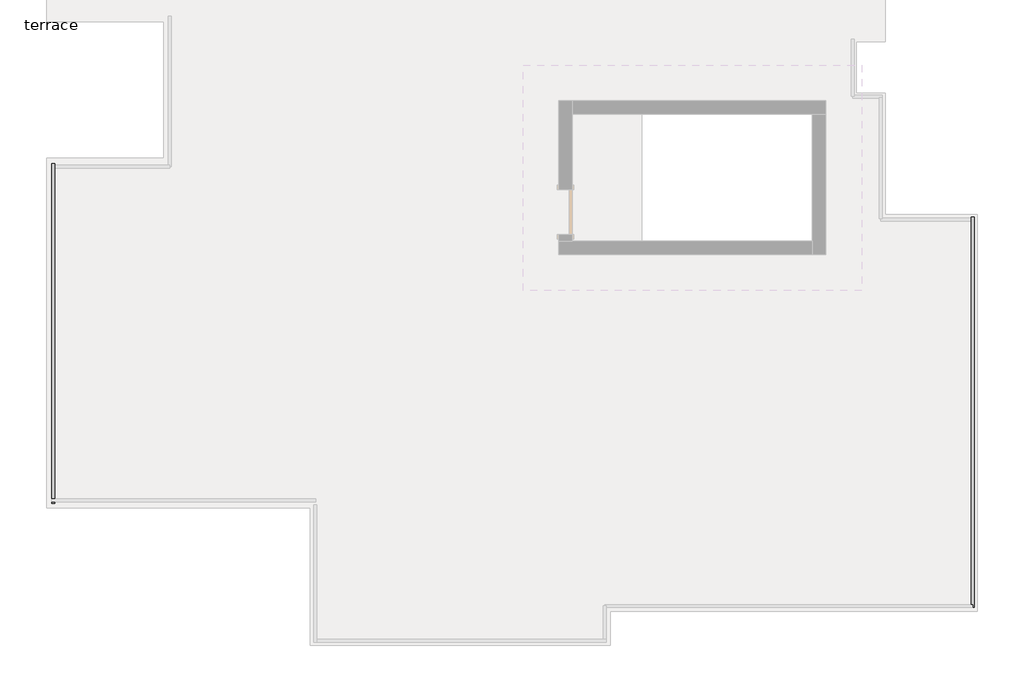
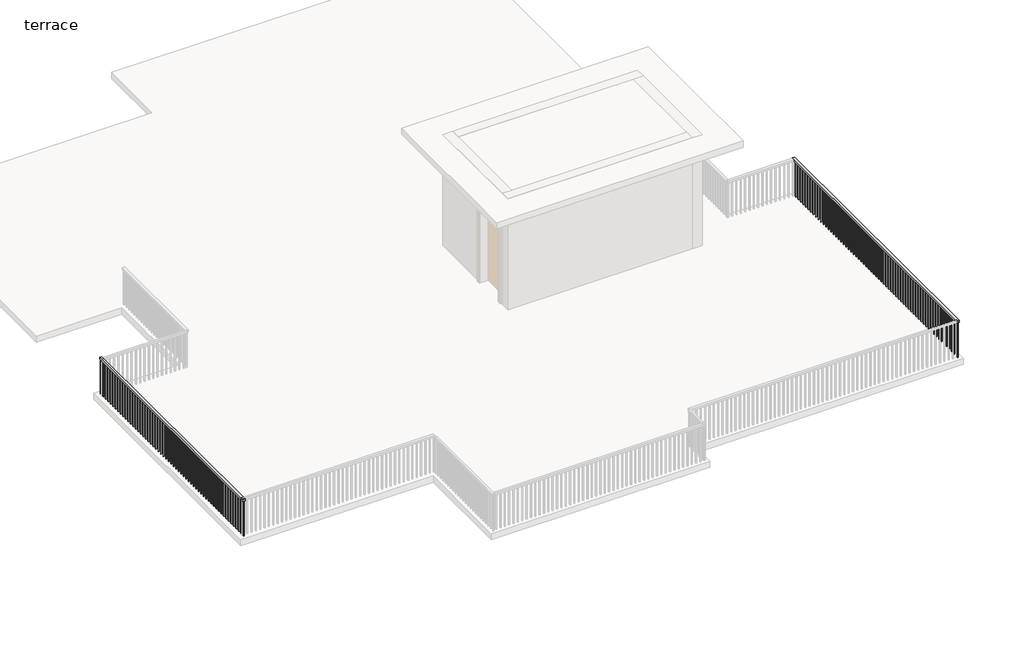
# One storey, part 3 of 7: 2 railings.
"""IFC4 building model written with IfcOpenShell, lengths in millimetres."""

from ifc_helpers import new_model, si_unit, frame, origin, place, context, project, spatial, polyline, outline, extrude, element, save

model = new_model("IFC4")

# Units and contexts
model_context = context("Model", 3, world=origin())
ifc_project = project(units=[si_unit("LENGTHUNIT", "METRE", prefix="MILLI")], contexts=[model_context])

# Site, building, storey
site = spatial("IfcSite", under=ifc_project)
building = spatial("IfcBuilding", under=site)
storey = spatial("IfcBuildingStorey", under=building, Name="terrace", Elevation=3810.0)

# Railings
placement = place(None, origin())
element("IfcRailing", 1, ObjectType="Handrail - Rectangular", at=placement, inside=storey, context=model_context, shape_type="SweptSolid", body=[
    extrude(outline(polyline([(1267.5109871, 2105.327622), (1318.3109871, 2105.327622), (1318.3109871, -4549.472378), (1267.5109871, -4549.472378), (1267.5109871, 2105.327622)])), frame((0.0, 0.0, 4673.6), z_axis=(0.0, 0.0, 1.0), x_axis=(1.0, 0.0, 0.0)), (0.0, 0.0, 1.0), 50.8),
    extrude(outline(polyline([(1283.3859871, -4489.147378), (1302.4359871, -4489.147378), (1302.4359871, -4508.197378), (1283.3859871, -4508.197378), (1283.3859871, -4489.147378)])), frame((0.0, 0.0, 3810.0), z_axis=(0.0, 0.0, 1.0), x_axis=(1.0, 0.0, 0.0)), (0.0, 0.0, 1.0), 863.6),
    extrude(outline(polyline([(1283.3859871, -4387.547378), (1302.4359871, -4387.547378), (1302.4359871, -4406.597378), (1283.3859871, -4406.597378), (1283.3859871, -4387.547378)])), frame((0.0, 0.0, 3810.0), z_axis=(0.0, 0.0, 1.0), x_axis=(1.0, 0.0, 0.0)), (0.0, 0.0, 1.0), 863.6),
    extrude(outline(polyline([(1283.3859871, -4285.947378), (1302.4359871, -4285.947378), (1302.4359871, -4304.997378), (1283.3859871, -4304.997378), (1283.3859871, -4285.947378)])), frame((0.0, 0.0, 3810.0), z_axis=(0.0, 0.0, 1.0), x_axis=(1.0, 0.0, 0.0)), (0.0, 0.0, 1.0), 863.6),
    extrude(outline(polyline([(1283.3859871, -4184.347378), (1302.4359871, -4184.347378), (1302.4359871, -4203.397378), (1283.3859871, -4203.397378), (1283.3859871, -4184.347378)])), frame((0.0, 0.0, 3810.0), z_axis=(0.0, 0.0, 1.0), x_axis=(1.0, 0.0, 0.0)), (0.0, 0.0, 1.0), 863.6),
    extrude(outline(polyline([(1283.3859871, -4082.747378), (1302.4359871, -4082.747378), (1302.4359871, -4101.797378), (1283.3859871, -4101.797378), (1283.3859871, -4082.747378)])), frame((0.0, 0.0, 3810.0), z_axis=(0.0, 0.0, 1.0), x_axis=(1.0, 0.0, 0.0)), (0.0, 0.0, 1.0), 863.6),
    extrude(outline(polyline([(1283.3859871, -3981.147378), (1302.4359871, -3981.147378), (1302.4359871, -4000.197378), (1283.3859871, -4000.197378), (1283.3859871, -3981.147378)])), frame((0.0, 0.0, 3810.0), z_axis=(0.0, 0.0, 1.0), x_axis=(1.0, 0.0, 0.0)), (0.0, 0.0, 1.0), 863.6),
    extrude(outline(polyline([(1283.3859871, -3879.547378), (1302.4359871, -3879.547378), (1302.4359871, -3898.597378), (1283.3859871, -3898.597378), (1283.3859871, -3879.547378)])), frame((0.0, 0.0, 3810.0), z_axis=(0.0, 0.0, 1.0), x_axis=(1.0, 0.0, 0.0)), (0.0, 0.0, 1.0), 863.6),
    extrude(outline(polyline([(1283.3859871, -3777.947378), (1302.4359871, -3777.947378), (1302.4359871, -3796.997378), (1283.3859871, -3796.997378), (1283.3859871, -3777.947378)])), frame((0.0, 0.0, 3810.0), z_axis=(0.0, 0.0, 1.0), x_axis=(1.0, 0.0, 0.0)), (0.0, 0.0, 1.0), 863.6),
    extrude(outline(polyline([(1283.3859871, -3676.347378), (1302.4359871, -3676.347378), (1302.4359871, -3695.397378), (1283.3859871, -3695.397378), (1283.3859871, -3676.347378)])), frame((0.0, 0.0, 3810.0), z_axis=(0.0, 0.0, 1.0), x_axis=(1.0, 0.0, 0.0)), (0.0, 0.0, 1.0), 863.6),
    extrude(outline(polyline([(1283.3859871, -3574.747378), (1302.4359871, -3574.747378), (1302.4359871, -3593.797378), (1283.3859871, -3593.797378), (1283.3859871, -3574.747378)])), frame((0.0, 0.0, 3810.0), z_axis=(0.0, 0.0, 1.0), x_axis=(1.0, 0.0, 0.0)), (0.0, 0.0, 1.0), 863.6),
    extrude(outline(polyline([(1283.3859871, -3473.147378), (1302.4359871, -3473.147378), (1302.4359871, -3492.197378), (1283.3859871, -3492.197378), (1283.3859871, -3473.147378)])), frame((0.0, 0.0, 3810.0), z_axis=(0.0, 0.0, 1.0), x_axis=(1.0, 0.0, 0.0)), (0.0, 0.0, 1.0), 863.6),
    extrude(outline(polyline([(1283.3859871, -3371.547378), (1302.4359871, -3371.547378), (1302.4359871, -3390.597378), (1283.3859871, -3390.597378), (1283.3859871, -3371.547378)])), frame((0.0, 0.0, 3810.0), z_axis=(0.0, 0.0, 1.0), x_axis=(1.0, 0.0, 0.0)), (0.0, 0.0, 1.0), 863.6),
    extrude(outline(polyline([(1283.3859871, -3269.947378), (1302.4359871, -3269.947378), (1302.4359871, -3288.997378), (1283.3859871, -3288.997378), (1283.3859871, -3269.947378)])), frame((0.0, 0.0, 3810.0), z_axis=(0.0, 0.0, 1.0), x_axis=(1.0, 0.0, 0.0)), (0.0, 0.0, 1.0), 863.6),
    extrude(outline(polyline([(1283.3859871, -3168.347378), (1302.4359871, -3168.347378), (1302.4359871, -3187.397378), (1283.3859871, -3187.397378), (1283.3859871, -3168.347378)])), frame((0.0, 0.0, 3810.0), z_axis=(0.0, 0.0, 1.0), x_axis=(1.0, 0.0, 0.0)), (0.0, 0.0, 1.0), 863.6),
    extrude(outline(polyline([(1283.3859871, -3066.747378), (1302.4359871, -3066.747378), (1302.4359871, -3085.797378), (1283.3859871, -3085.797378), (1283.3859871, -3066.747378)])), frame((0.0, 0.0, 3810.0), z_axis=(0.0, 0.0, 1.0), x_axis=(1.0, 0.0, 0.0)), (0.0, 0.0, 1.0), 863.6),
    extrude(outline(polyline([(1283.3859871, -2965.147378), (1302.4359871, -2965.147378), (1302.4359871, -2984.197378), (1283.3859871, -2984.197378), (1283.3859871, -2965.147378)])), frame((0.0, 0.0, 3810.0), z_axis=(0.0, 0.0, 1.0), x_axis=(1.0, 0.0, 0.0)), (0.0, 0.0, 1.0), 863.6),
    extrude(outline(polyline([(1283.3859871, -2863.547378), (1302.4359871, -2863.547378), (1302.4359871, -2882.597378), (1283.3859871, -2882.597378), (1283.3859871, -2863.547378)])), frame((0.0, 0.0, 3810.0), z_axis=(0.0, 0.0, 1.0), x_axis=(1.0, 0.0, 0.0)), (0.0, 0.0, 1.0), 863.6),
    extrude(outline(polyline([(1283.3859871, -2761.947378), (1302.4359871, -2761.947378), (1302.4359871, -2780.997378), (1283.3859871, -2780.997378), (1283.3859871, -2761.947378)])), frame((0.0, 0.0, 3810.0), z_axis=(0.0, 0.0, 1.0), x_axis=(1.0, 0.0, 0.0)), (0.0, 0.0, 1.0), 863.6),
    extrude(outline(polyline([(1283.3859871, -2660.347378), (1302.4359871, -2660.347378), (1302.4359871, -2679.397378), (1283.3859871, -2679.397378), (1283.3859871, -2660.347378)])), frame((0.0, 0.0, 3810.0), z_axis=(0.0, 0.0, 1.0), x_axis=(1.0, 0.0, 0.0)), (0.0, 0.0, 1.0), 863.6),
    extrude(outline(polyline([(1283.3859871, -2558.747378), (1302.4359871, -2558.747378), (1302.4359871, -2577.797378), (1283.3859871, -2577.797378), (1283.3859871, -2558.747378)])), frame((0.0, 0.0, 3810.0), z_axis=(0.0, 0.0, 1.0), x_axis=(1.0, 0.0, 0.0)), (0.0, 0.0, 1.0), 863.6),
    extrude(outline(polyline([(1283.3859871, -2457.147378), (1302.4359871, -2457.147378), (1302.4359871, -2476.197378), (1283.3859871, -2476.197378), (1283.3859871, -2457.147378)])), frame((0.0, 0.0, 3810.0), z_axis=(0.0, 0.0, 1.0), x_axis=(1.0, 0.0, 0.0)), (0.0, 0.0, 1.0), 863.6),
    extrude(outline(polyline([(1283.3859871, -2355.547378), (1302.4359871, -2355.547378), (1302.4359871, -2374.597378), (1283.3859871, -2374.597378), (1283.3859871, -2355.547378)])), frame((0.0, 0.0, 3810.0), z_axis=(0.0, 0.0, 1.0), x_axis=(1.0, 0.0, 0.0)), (0.0, 0.0, 1.0), 863.6),
    extrude(outline(polyline([(1283.3859871, -2253.947378), (1302.4359871, -2253.947378), (1302.4359871, -2272.997378), (1283.3859871, -2272.997378), (1283.3859871, -2253.947378)])), frame((0.0, 0.0, 3810.0), z_axis=(0.0, 0.0, 1.0), x_axis=(1.0, 0.0, 0.0)), (0.0, 0.0, 1.0), 863.6),
    extrude(outline(polyline([(1283.3859871, -2152.347378), (1302.4359871, -2152.347378), (1302.4359871, -2171.397378), (1283.3859871, -2171.397378), (1283.3859871, -2152.347378)])), frame((0.0, 0.0, 3810.0), z_axis=(0.0, 0.0, 1.0), x_axis=(1.0, 0.0, 0.0)), (0.0, 0.0, 1.0), 863.6),
    extrude(outline(polyline([(1283.3859871, -2050.747378), (1302.4359871, -2050.747378), (1302.4359871, -2069.797378), (1283.3859871, -2069.797378), (1283.3859871, -2050.747378)])), frame((0.0, 0.0, 3810.0), z_axis=(0.0, 0.0, 1.0), x_axis=(1.0, 0.0, 0.0)), (0.0, 0.0, 1.0), 863.6),
    extrude(outline(polyline([(1283.3859871, -1949.147378), (1302.4359871, -1949.147378), (1302.4359871, -1968.197378), (1283.3859871, -1968.197378), (1283.3859871, -1949.147378)])), frame((0.0, 0.0, 3810.0), z_axis=(0.0, 0.0, 1.0), x_axis=(1.0, 0.0, 0.0)), (0.0, 0.0, 1.0), 863.6),
    extrude(outline(polyline([(1283.3859871, -1847.547378), (1302.4359871, -1847.547378), (1302.4359871, -1866.597378), (1283.3859871, -1866.597378), (1283.3859871, -1847.547378)])), frame((0.0, 0.0, 3810.0), z_axis=(0.0, 0.0, 1.0), x_axis=(1.0, 0.0, 0.0)), (0.0, 0.0, 1.0), 863.6),
    extrude(outline(polyline([(1283.3859871, -1745.947378), (1302.4359871, -1745.947378), (1302.4359871, -1764.997378), (1283.3859871, -1764.997378), (1283.3859871, -1745.947378)])), frame((0.0, 0.0, 3810.0), z_axis=(0.0, 0.0, 1.0), x_axis=(1.0, 0.0, 0.0)), (0.0, 0.0, 1.0), 863.6),
    extrude(outline(polyline([(1283.3859871, -1644.347378), (1302.4359871, -1644.347378), (1302.4359871, -1663.397378), (1283.3859871, -1663.397378), (1283.3859871, -1644.347378)])), frame((0.0, 0.0, 3810.0), z_axis=(0.0, 0.0, 1.0), x_axis=(1.0, 0.0, 0.0)), (0.0, 0.0, 1.0), 863.6),
    extrude(outline(polyline([(1283.3859871, -1542.747378), (1302.4359871, -1542.747378), (1302.4359871, -1561.797378), (1283.3859871, -1561.797378), (1283.3859871, -1542.747378)])), frame((0.0, 0.0, 3810.0), z_axis=(0.0, 0.0, 1.0), x_axis=(1.0, 0.0, 0.0)), (0.0, 0.0, 1.0), 863.6),
    extrude(outline(polyline([(1283.3859871, -1441.147378), (1302.4359871, -1441.147378), (1302.4359871, -1460.197378), (1283.3859871, -1460.197378), (1283.3859871, -1441.147378)])), frame((0.0, 0.0, 3810.0), z_axis=(0.0, 0.0, 1.0), x_axis=(1.0, 0.0, 0.0)), (0.0, 0.0, 1.0), 863.6),
    extrude(outline(polyline([(1283.3859871, -1339.547378), (1302.4359871, -1339.547378), (1302.4359871, -1358.597378), (1283.3859871, -1358.597378), (1283.3859871, -1339.547378)])), frame((0.0, 0.0, 3810.0), z_axis=(0.0, 0.0, 1.0), x_axis=(1.0, 0.0, 0.0)), (0.0, 0.0, 1.0), 863.6),
    extrude(outline(polyline([(1283.3859871, -1237.947378), (1302.4359871, -1237.947378), (1302.4359871, -1256.997378), (1283.3859871, -1256.997378), (1283.3859871, -1237.947378)])), frame((0.0, 0.0, 3810.0), z_axis=(0.0, 0.0, 1.0), x_axis=(1.0, 0.0, 0.0)), (0.0, 0.0, 1.0), 863.6),
    extrude(outline(polyline([(1283.3859871, -1136.347378), (1302.4359871, -1136.347378), (1302.4359871, -1155.397378), (1283.3859871, -1155.397378), (1283.3859871, -1136.347378)])), frame((0.0, 0.0, 3810.0), z_axis=(0.0, 0.0, 1.0), x_axis=(1.0, 0.0, 0.0)), (0.0, 0.0, 1.0), 863.6),
    extrude(outline(polyline([(1283.3859871, -1034.747378), (1302.4359871, -1034.747378), (1302.4359871, -1053.797378), (1283.3859871, -1053.797378), (1283.3859871, -1034.747378)])), frame((0.0, 0.0, 3810.0), z_axis=(0.0, 0.0, 1.0), x_axis=(1.0, 0.0, 0.0)), (0.0, 0.0, 1.0), 863.6),
    extrude(outline(polyline([(1283.3859871, -933.147378), (1302.4359871, -933.147378), (1302.4359871, -952.197378), (1283.3859871, -952.197378), (1283.3859871, -933.147378)])), frame((0.0, 0.0, 3810.0), z_axis=(0.0, 0.0, 1.0), x_axis=(1.0, 0.0, 0.0)), (0.0, 0.0, 1.0), 863.6),
    extrude(outline(polyline([(1283.3859871, -831.547378), (1302.4359871, -831.547378), (1302.4359871, -850.597378), (1283.3859871, -850.597378), (1283.3859871, -831.547378)])), frame((0.0, 0.0, 3810.0), z_axis=(0.0, 0.0, 1.0), x_axis=(1.0, 0.0, 0.0)), (0.0, 0.0, 1.0), 863.6),
    extrude(outline(polyline([(1283.3859871, -729.947378), (1302.4359871, -729.947378), (1302.4359871, -748.997378), (1283.3859871, -748.997378), (1283.3859871, -729.947378)])), frame((0.0, 0.0, 3810.0), z_axis=(0.0, 0.0, 1.0), x_axis=(1.0, 0.0, 0.0)), (0.0, 0.0, 1.0), 863.6),
    extrude(outline(polyline([(1283.3859871, -628.347378), (1302.4359871, -628.347378), (1302.4359871, -647.397378), (1283.3859871, -647.397378), (1283.3859871, -628.347378)])), frame((0.0, 0.0, 3810.0), z_axis=(0.0, 0.0, 1.0), x_axis=(1.0, 0.0, 0.0)), (0.0, 0.0, 1.0), 863.6),
    extrude(outline(polyline([(1283.3859871, -526.747378), (1302.4359871, -526.747378), (1302.4359871, -545.797378), (1283.3859871, -545.797378), (1283.3859871, -526.747378)])), frame((0.0, 0.0, 3810.0), z_axis=(0.0, 0.0, 1.0), x_axis=(1.0, 0.0, 0.0)), (0.0, 0.0, 1.0), 863.6),
    extrude(outline(polyline([(1283.3859871, -425.147378), (1302.4359871, -425.147378), (1302.4359871, -444.197378), (1283.3859871, -444.197378), (1283.3859871, -425.147378)])), frame((0.0, 0.0, 3810.0), z_axis=(0.0, 0.0, 1.0), x_axis=(1.0, 0.0, 0.0)), (0.0, 0.0, 1.0), 863.6),
    extrude(outline(polyline([(1283.3859871, -323.547378), (1302.4359871, -323.547378), (1302.4359871, -342.597378), (1283.3859871, -342.597378), (1283.3859871, -323.547378)])), frame((0.0, 0.0, 3810.0), z_axis=(0.0, 0.0, 1.0), x_axis=(1.0, 0.0, 0.0)), (0.0, 0.0, 1.0), 863.6),
    extrude(outline(polyline([(1283.3859871, -221.947378), (1302.4359871, -221.947378), (1302.4359871, -240.997378), (1283.3859871, -240.997378), (1283.3859871, -221.947378)])), frame((0.0, 0.0, 3810.0), z_axis=(0.0, 0.0, 1.0), x_axis=(1.0, 0.0, 0.0)), (0.0, 0.0, 1.0), 863.6),
    extrude(outline(polyline([(1283.3859871, -120.347378), (1302.4359871, -120.347378), (1302.4359871, -139.397378), (1283.3859871, -139.397378), (1283.3859871, -120.347378)])), frame((0.0, 0.0, 3810.0), z_axis=(0.0, 0.0, 1.0), x_axis=(1.0, 0.0, 0.0)), (0.0, 0.0, 1.0), 863.6),
    extrude(outline(polyline([(1283.3859871, -18.747378), (1302.4359871, -18.747378), (1302.4359871, -37.797378), (1283.3859871, -37.797378), (1283.3859871, -18.747378)])), frame((0.0, 0.0, 3810.0), z_axis=(0.0, 0.0, 1.0), x_axis=(1.0, 0.0, 0.0)), (0.0, 0.0, 1.0), 863.6),
    extrude(outline(polyline([(1283.3859871, 82.852622), (1302.4359871, 82.852622), (1302.4359871, 63.802622), (1283.3859871, 63.802622), (1283.3859871, 82.852622)])), frame((0.0, 0.0, 3810.0), z_axis=(0.0, 0.0, 1.0), x_axis=(1.0, 0.0, 0.0)), (0.0, 0.0, 1.0), 863.6),
    extrude(outline(polyline([(1283.3859871, 184.452622), (1302.4359871, 184.452622), (1302.4359871, 165.402622), (1283.3859871, 165.402622), (1283.3859871, 184.452622)])), frame((0.0, 0.0, 3810.0), z_axis=(0.0, 0.0, 1.0), x_axis=(1.0, 0.0, 0.0)), (0.0, 0.0, 1.0), 863.6),
    extrude(outline(polyline([(1283.3859871, 286.052622), (1302.4359871, 286.052622), (1302.4359871, 267.002622), (1283.3859871, 267.002622), (1283.3859871, 286.052622)])), frame((0.0, 0.0, 3810.0), z_axis=(0.0, 0.0, 1.0), x_axis=(1.0, 0.0, 0.0)), (0.0, 0.0, 1.0), 863.6),
    extrude(outline(polyline([(1283.3859871, 387.652622), (1302.4359871, 387.652622), (1302.4359871, 368.602622), (1283.3859871, 368.602622), (1283.3859871, 387.652622)])), frame((0.0, 0.0, 3810.0), z_axis=(0.0, 0.0, 1.0), x_axis=(1.0, 0.0, 0.0)), (0.0, 0.0, 1.0), 863.6),
    extrude(outline(polyline([(1283.3859871, 489.252622), (1302.4359871, 489.252622), (1302.4359871, 470.202622), (1283.3859871, 470.202622), (1283.3859871, 489.252622)])), frame((0.0, 0.0, 3810.0), z_axis=(0.0, 0.0, 1.0), x_axis=(1.0, 0.0, 0.0)), (0.0, 0.0, 1.0), 863.6),
    extrude(outline(polyline([(1283.3859871, 590.852622), (1302.4359871, 590.852622), (1302.4359871, 571.802622), (1283.3859871, 571.802622), (1283.3859871, 590.852622)])), frame((0.0, 0.0, 3810.0), z_axis=(0.0, 0.0, 1.0), x_axis=(1.0, 0.0, 0.0)), (0.0, 0.0, 1.0), 863.6),
    extrude(outline(polyline([(1283.3859871, 692.452622), (1302.4359871, 692.452622), (1302.4359871, 673.402622), (1283.3859871, 673.402622), (1283.3859871, 692.452622)])), frame((0.0, 0.0, 3810.0), z_axis=(0.0, 0.0, 1.0), x_axis=(1.0, 0.0, 0.0)), (0.0, 0.0, 1.0), 863.6),
    extrude(outline(polyline([(1283.3859871, 794.052622), (1302.4359871, 794.052622), (1302.4359871, 775.002622), (1283.3859871, 775.002622), (1283.3859871, 794.052622)])), frame((0.0, 0.0, 3810.0), z_axis=(0.0, 0.0, 1.0), x_axis=(1.0, 0.0, 0.0)), (0.0, 0.0, 1.0), 863.6),
    extrude(outline(polyline([(1283.3859871, 895.652622), (1302.4359871, 895.652622), (1302.4359871, 876.602622), (1283.3859871, 876.602622), (1283.3859871, 895.652622)])), frame((0.0, 0.0, 3810.0), z_axis=(0.0, 0.0, 1.0), x_axis=(1.0, 0.0, 0.0)), (0.0, 0.0, 1.0), 863.6),
    extrude(outline(polyline([(1283.3859871, 997.252622), (1302.4359871, 997.252622), (1302.4359871, 978.202622), (1283.3859871, 978.202622), (1283.3859871, 997.252622)])), frame((0.0, 0.0, 3810.0), z_axis=(0.0, 0.0, 1.0), x_axis=(1.0, 0.0, 0.0)), (0.0, 0.0, 1.0), 863.6),
    extrude(outline(polyline([(1283.3859871, 1098.852622), (1302.4359871, 1098.852622), (1302.4359871, 1079.802622), (1283.3859871, 1079.802622), (1283.3859871, 1098.852622)])), frame((0.0, 0.0, 3810.0), z_axis=(0.0, 0.0, 1.0), x_axis=(1.0, 0.0, 0.0)), (0.0, 0.0, 1.0), 863.6),
    extrude(outline(polyline([(1283.3859871, 1200.452622), (1302.4359871, 1200.452622), (1302.4359871, 1181.402622), (1283.3859871, 1181.402622), (1283.3859871, 1200.452622)])), frame((0.0, 0.0, 3810.0), z_axis=(0.0, 0.0, 1.0), x_axis=(1.0, 0.0, 0.0)), (0.0, 0.0, 1.0), 863.6),
    extrude(outline(polyline([(1283.3859871, 1302.052622), (1302.4359871, 1302.052622), (1302.4359871, 1283.002622), (1283.3859871, 1283.002622), (1283.3859871, 1302.052622)])), frame((0.0, 0.0, 3810.0), z_axis=(0.0, 0.0, 1.0), x_axis=(1.0, 0.0, 0.0)), (0.0, 0.0, 1.0), 863.6),
    extrude(outline(polyline([(1283.3859871, 1403.652622), (1302.4359871, 1403.652622), (1302.4359871, 1384.602622), (1283.3859871, 1384.602622), (1283.3859871, 1403.652622)])), frame((0.0, 0.0, 3810.0), z_axis=(0.0, 0.0, 1.0), x_axis=(1.0, 0.0, 0.0)), (0.0, 0.0, 1.0), 863.6),
    extrude(outline(polyline([(1283.3859871, 1505.252622), (1302.4359871, 1505.252622), (1302.4359871, 1486.202622), (1283.3859871, 1486.202622), (1283.3859871, 1505.252622)])), frame((0.0, 0.0, 3810.0), z_axis=(0.0, 0.0, 1.0), x_axis=(1.0, 0.0, 0.0)), (0.0, 0.0, 1.0), 863.6),
    extrude(outline(polyline([(1283.3859871, 1606.852622), (1302.4359871, 1606.852622), (1302.4359871, 1587.802622), (1283.3859871, 1587.802622), (1283.3859871, 1606.852622)])), frame((0.0, 0.0, 3810.0), z_axis=(0.0, 0.0, 1.0), x_axis=(1.0, 0.0, 0.0)), (0.0, 0.0, 1.0), 863.6),
    extrude(outline(polyline([(1283.3859871, 1708.452622), (1302.4359871, 1708.452622), (1302.4359871, 1689.402622), (1283.3859871, 1689.402622), (1283.3859871, 1708.452622)])), frame((0.0, 0.0, 3810.0), z_axis=(0.0, 0.0, 1.0), x_axis=(1.0, 0.0, 0.0)), (0.0, 0.0, 1.0), 863.6),
    extrude(outline(polyline([(1283.3859871, 1810.052622), (1302.4359871, 1810.052622), (1302.4359871, 1791.002622), (1283.3859871, 1791.002622), (1283.3859871, 1810.052622)])), frame((0.0, 0.0, 3810.0), z_axis=(0.0, 0.0, 1.0), x_axis=(1.0, 0.0, 0.0)), (0.0, 0.0, 1.0), 863.6),
    extrude(outline(polyline([(1283.3859871, 1911.652622), (1302.4359871, 1911.652622), (1302.4359871, 1892.602622), (1283.3859871, 1892.602622), (1283.3859871, 1911.652622)])), frame((0.0, 0.0, 3810.0), z_axis=(0.0, 0.0, 1.0), x_axis=(1.0, 0.0, 0.0)), (0.0, 0.0, 1.0), 863.6),
    extrude(outline(polyline([(1283.3859871, 2013.252622), (1302.4359871, 2013.252622), (1302.4359871, 1994.202622), (1283.3859871, 1994.202622), (1283.3859871, 2013.252622)])), frame((0.0, 0.0, 3810.0), z_axis=(0.0, 0.0, 1.0), x_axis=(1.0, 0.0, 0.0)), (0.0, 0.0, 1.0), 863.6),
    extrude(outline(polyline([(1283.3859871, -4530.422378), (1302.4359871, -4530.422378), (1302.4359871, -4549.472378), (1283.3859871, -4549.472378), (1283.3859871, -4530.422378)])), frame((0.0, 0.0, 3810.0), z_axis=(0.0, 0.0, 1.0), x_axis=(1.0, 0.0, 0.0)), (0.0, 0.0, 1.0), 863.6),
    extrude(outline(polyline([(1283.3859871, 2105.327622), (1302.4359871, 2105.327622), (1302.4359871, 2086.277622), (1283.3859871, 2086.277622), (1283.3859871, 2105.327622)])), frame((0.0, 0.0, 3810.0), z_axis=(0.0, 0.0, 1.0), x_axis=(1.0, 0.0, 0.0)), (0.0, 0.0, 1.0), 863.6),
])
element("IfcRailing", 2, ObjectType="Handrail - Rectangular", at=placement, inside=storey, context=model_context, shape_type="SweptSolid", body=[
    extrude(outline(polyline([(-14340.7890129, -2777.822378), (-14391.5890129, -2777.822378), (-14391.5890129, 3013.377622), (-14340.7890129, 3013.377622), (-14340.7890129, -2777.822378)])), frame((0.0, 0.0, 4673.6), z_axis=(0.0, 0.0, 1.0), x_axis=(1.0, 0.0, 0.0)), (0.0, 0.0, 1.0), 50.8),
    extrude(outline(polyline([(-14356.6640129, 2902.252622), (-14375.7140129, 2902.252622), (-14375.7140129, 2921.302622), (-14356.6640129, 2921.302622), (-14356.6640129, 2902.252622)])), frame((0.0, 0.0, 3810.0), z_axis=(0.0, 0.0, 1.0), x_axis=(1.0, 0.0, 0.0)), (0.0, 0.0, 1.0), 863.6),
    extrude(outline(polyline([(-14356.6640129, 2800.652622), (-14375.7140129, 2800.652622), (-14375.7140129, 2819.702622), (-14356.6640129, 2819.702622), (-14356.6640129, 2800.652622)])), frame((0.0, 0.0, 3810.0), z_axis=(0.0, 0.0, 1.0), x_axis=(1.0, 0.0, 0.0)), (0.0, 0.0, 1.0), 863.6),
    extrude(outline(polyline([(-14356.6640129, 2699.052622), (-14375.7140129, 2699.052622), (-14375.7140129, 2718.102622), (-14356.6640129, 2718.102622), (-14356.6640129, 2699.052622)])), frame((0.0, 0.0, 3810.0), z_axis=(0.0, 0.0, 1.0), x_axis=(1.0, 0.0, 0.0)), (0.0, 0.0, 1.0), 863.6),
    extrude(outline(polyline([(-14356.6640129, 2597.452622), (-14375.7140129, 2597.452622), (-14375.7140129, 2616.502622), (-14356.6640129, 2616.502622), (-14356.6640129, 2597.452622)])), frame((0.0, 0.0, 3810.0), z_axis=(0.0, 0.0, 1.0), x_axis=(1.0, 0.0, 0.0)), (0.0, 0.0, 1.0), 863.6),
    extrude(outline(polyline([(-14356.6640129, 2495.852622), (-14375.7140129, 2495.852622), (-14375.7140129, 2514.902622), (-14356.6640129, 2514.902622), (-14356.6640129, 2495.852622)])), frame((0.0, 0.0, 3810.0), z_axis=(0.0, 0.0, 1.0), x_axis=(1.0, 0.0, 0.0)), (0.0, 0.0, 1.0), 863.6),
    extrude(outline(polyline([(-14356.6640129, 2394.252622), (-14375.7140129, 2394.252622), (-14375.7140129, 2413.302622), (-14356.6640129, 2413.302622), (-14356.6640129, 2394.252622)])), frame((0.0, 0.0, 3810.0), z_axis=(0.0, 0.0, 1.0), x_axis=(1.0, 0.0, 0.0)), (0.0, 0.0, 1.0), 863.6),
    extrude(outline(polyline([(-14356.6640129, 2292.652622), (-14375.7140129, 2292.652622), (-14375.7140129, 2311.702622), (-14356.6640129, 2311.702622), (-14356.6640129, 2292.652622)])), frame((0.0, 0.0, 3810.0), z_axis=(0.0, 0.0, 1.0), x_axis=(1.0, 0.0, 0.0)), (0.0, 0.0, 1.0), 863.6),
    extrude(outline(polyline([(-14356.6640129, 2191.052622), (-14375.7140129, 2191.052622), (-14375.7140129, 2210.102622), (-14356.6640129, 2210.102622), (-14356.6640129, 2191.052622)])), frame((0.0, 0.0, 3810.0), z_axis=(0.0, 0.0, 1.0), x_axis=(1.0, 0.0, 0.0)), (0.0, 0.0, 1.0), 863.6),
    extrude(outline(polyline([(-14356.6640129, 2089.452622), (-14375.7140129, 2089.452622), (-14375.7140129, 2108.502622), (-14356.6640129, 2108.502622), (-14356.6640129, 2089.452622)])), frame((0.0, 0.0, 3810.0), z_axis=(0.0, 0.0, 1.0), x_axis=(1.0, 0.0, 0.0)), (0.0, 0.0, 1.0), 863.6),
    extrude(outline(polyline([(-14356.6640129, 1987.852622), (-14375.7140129, 1987.852622), (-14375.7140129, 2006.902622), (-14356.6640129, 2006.902622), (-14356.6640129, 1987.852622)])), frame((0.0, 0.0, 3810.0), z_axis=(0.0, 0.0, 1.0), x_axis=(1.0, 0.0, 0.0)), (0.0, 0.0, 1.0), 863.6),
    extrude(outline(polyline([(-14356.6640129, 1886.252622), (-14375.7140129, 1886.252622), (-14375.7140129, 1905.302622), (-14356.6640129, 1905.302622), (-14356.6640129, 1886.252622)])), frame((0.0, 0.0, 3810.0), z_axis=(0.0, 0.0, 1.0), x_axis=(1.0, 0.0, 0.0)), (0.0, 0.0, 1.0), 863.6),
    extrude(outline(polyline([(-14356.6640129, 1784.652622), (-14375.7140129, 1784.652622), (-14375.7140129, 1803.702622), (-14356.6640129, 1803.702622), (-14356.6640129, 1784.652622)])), frame((0.0, 0.0, 3810.0), z_axis=(0.0, 0.0, 1.0), x_axis=(1.0, 0.0, 0.0)), (0.0, 0.0, 1.0), 863.6),
    extrude(outline(polyline([(-14356.6640129, 1683.052622), (-14375.7140129, 1683.052622), (-14375.7140129, 1702.102622), (-14356.6640129, 1702.102622), (-14356.6640129, 1683.052622)])), frame((0.0, 0.0, 3810.0), z_axis=(0.0, 0.0, 1.0), x_axis=(1.0, 0.0, 0.0)), (0.0, 0.0, 1.0), 863.6),
    extrude(outline(polyline([(-14356.6640129, 1581.452622), (-14375.7140129, 1581.452622), (-14375.7140129, 1600.502622), (-14356.6640129, 1600.502622), (-14356.6640129, 1581.452622)])), frame((0.0, 0.0, 3810.0), z_axis=(0.0, 0.0, 1.0), x_axis=(1.0, 0.0, 0.0)), (0.0, 0.0, 1.0), 863.6),
    extrude(outline(polyline([(-14356.6640129, 1479.852622), (-14375.7140129, 1479.852622), (-14375.7140129, 1498.902622), (-14356.6640129, 1498.902622), (-14356.6640129, 1479.852622)])), frame((0.0, 0.0, 3810.0), z_axis=(0.0, 0.0, 1.0), x_axis=(1.0, 0.0, 0.0)), (0.0, 0.0, 1.0), 863.6),
    extrude(outline(polyline([(-14356.6640129, 1378.252622), (-14375.7140129, 1378.252622), (-14375.7140129, 1397.302622), (-14356.6640129, 1397.302622), (-14356.6640129, 1378.252622)])), frame((0.0, 0.0, 3810.0), z_axis=(0.0, 0.0, 1.0), x_axis=(1.0, 0.0, 0.0)), (0.0, 0.0, 1.0), 863.6),
    extrude(outline(polyline([(-14356.6640129, 1276.652622), (-14375.7140129, 1276.652622), (-14375.7140129, 1295.702622), (-14356.6640129, 1295.702622), (-14356.6640129, 1276.652622)])), frame((0.0, 0.0, 3810.0), z_axis=(0.0, 0.0, 1.0), x_axis=(1.0, 0.0, 0.0)), (0.0, 0.0, 1.0), 863.6),
    extrude(outline(polyline([(-14356.6640129, 1175.052622), (-14375.7140129, 1175.052622), (-14375.7140129, 1194.102622), (-14356.6640129, 1194.102622), (-14356.6640129, 1175.052622)])), frame((0.0, 0.0, 3810.0), z_axis=(0.0, 0.0, 1.0), x_axis=(1.0, 0.0, 0.0)), (0.0, 0.0, 1.0), 863.6),
    extrude(outline(polyline([(-14356.6640129, 1073.452622), (-14375.7140129, 1073.452622), (-14375.7140129, 1092.502622), (-14356.6640129, 1092.502622), (-14356.6640129, 1073.452622)])), frame((0.0, 0.0, 3810.0), z_axis=(0.0, 0.0, 1.0), x_axis=(1.0, 0.0, 0.0)), (0.0, 0.0, 1.0), 863.6),
    extrude(outline(polyline([(-14356.6640129, 971.852622), (-14375.7140129, 971.852622), (-14375.7140129, 990.902622), (-14356.6640129, 990.902622), (-14356.6640129, 971.852622)])), frame((0.0, 0.0, 3810.0), z_axis=(0.0, 0.0, 1.0), x_axis=(1.0, 0.0, 0.0)), (0.0, 0.0, 1.0), 863.6),
    extrude(outline(polyline([(-14356.6640129, 870.252622), (-14375.7140129, 870.252622), (-14375.7140129, 889.302622), (-14356.6640129, 889.302622), (-14356.6640129, 870.252622)])), frame((0.0, 0.0, 3810.0), z_axis=(0.0, 0.0, 1.0), x_axis=(1.0, 0.0, 0.0)), (0.0, 0.0, 1.0), 863.6),
    extrude(outline(polyline([(-14356.6640129, 768.652622), (-14375.7140129, 768.652622), (-14375.7140129, 787.702622), (-14356.6640129, 787.702622), (-14356.6640129, 768.652622)])), frame((0.0, 0.0, 3810.0), z_axis=(0.0, 0.0, 1.0), x_axis=(1.0, 0.0, 0.0)), (0.0, 0.0, 1.0), 863.6),
    extrude(outline(polyline([(-14356.6640129, 667.052622), (-14375.7140129, 667.052622), (-14375.7140129, 686.102622), (-14356.6640129, 686.102622), (-14356.6640129, 667.052622)])), frame((0.0, 0.0, 3810.0), z_axis=(0.0, 0.0, 1.0), x_axis=(1.0, 0.0, 0.0)), (0.0, 0.0, 1.0), 863.6),
    extrude(outline(polyline([(-14356.6640129, 565.452622), (-14375.7140129, 565.452622), (-14375.7140129, 584.502622), (-14356.6640129, 584.502622), (-14356.6640129, 565.452622)])), frame((0.0, 0.0, 3810.0), z_axis=(0.0, 0.0, 1.0), x_axis=(1.0, 0.0, 0.0)), (0.0, 0.0, 1.0), 863.6),
    extrude(outline(polyline([(-14356.6640129, 463.852622), (-14375.7140129, 463.852622), (-14375.7140129, 482.902622), (-14356.6640129, 482.902622), (-14356.6640129, 463.852622)])), frame((0.0, 0.0, 3810.0), z_axis=(0.0, 0.0, 1.0), x_axis=(1.0, 0.0, 0.0)), (0.0, 0.0, 1.0), 863.6),
    extrude(outline(polyline([(-14356.6640129, 362.252622), (-14375.7140129, 362.252622), (-14375.7140129, 381.302622), (-14356.6640129, 381.302622), (-14356.6640129, 362.252622)])), frame((0.0, 0.0, 3810.0), z_axis=(0.0, 0.0, 1.0), x_axis=(1.0, 0.0, 0.0)), (0.0, 0.0, 1.0), 863.6),
    extrude(outline(polyline([(-14356.6640129, 260.652622), (-14375.7140129, 260.652622), (-14375.7140129, 279.702622), (-14356.6640129, 279.702622), (-14356.6640129, 260.652622)])), frame((0.0, 0.0, 3810.0), z_axis=(0.0, 0.0, 1.0), x_axis=(1.0, 0.0, 0.0)), (0.0, 0.0, 1.0), 863.6),
    extrude(outline(polyline([(-14356.6640129, 159.052622), (-14375.7140129, 159.052622), (-14375.7140129, 178.102622), (-14356.6640129, 178.102622), (-14356.6640129, 159.052622)])), frame((0.0, 0.0, 3810.0), z_axis=(0.0, 0.0, 1.0), x_axis=(1.0, 0.0, 0.0)), (0.0, 0.0, 1.0), 863.6),
    extrude(outline(polyline([(-14356.6640129, 57.452622), (-14375.7140129, 57.452622), (-14375.7140129, 76.502622), (-14356.6640129, 76.502622), (-14356.6640129, 57.452622)])), frame((0.0, 0.0, 3810.0), z_axis=(0.0, 0.0, 1.0), x_axis=(1.0, 0.0, 0.0)), (0.0, 0.0, 1.0), 863.6),
    extrude(outline(polyline([(-14356.6640129, -44.147378), (-14375.7140129, -44.147378), (-14375.7140129, -25.097378), (-14356.6640129, -25.097378), (-14356.6640129, -44.147378)])), frame((0.0, 0.0, 3810.0), z_axis=(0.0, 0.0, 1.0), x_axis=(1.0, 0.0, 0.0)), (0.0, 0.0, 1.0), 863.6),
    extrude(outline(polyline([(-14356.6640129, -145.747378), (-14375.7140129, -145.747378), (-14375.7140129, -126.697378), (-14356.6640129, -126.697378), (-14356.6640129, -145.747378)])), frame((0.0, 0.0, 3810.0), z_axis=(0.0, 0.0, 1.0), x_axis=(1.0, 0.0, 0.0)), (0.0, 0.0, 1.0), 863.6),
    extrude(outline(polyline([(-14356.6640129, -247.347378), (-14375.7140129, -247.347378), (-14375.7140129, -228.297378), (-14356.6640129, -228.297378), (-14356.6640129, -247.347378)])), frame((0.0, 0.0, 3810.0), z_axis=(0.0, 0.0, 1.0), x_axis=(1.0, 0.0, 0.0)), (0.0, 0.0, 1.0), 863.6),
    extrude(outline(polyline([(-14356.6640129, -348.947378), (-14375.7140129, -348.947378), (-14375.7140129, -329.897378), (-14356.6640129, -329.897378), (-14356.6640129, -348.947378)])), frame((0.0, 0.0, 3810.0), z_axis=(0.0, 0.0, 1.0), x_axis=(1.0, 0.0, 0.0)), (0.0, 0.0, 1.0), 863.6),
    extrude(outline(polyline([(-14356.6640129, -450.547378), (-14375.7140129, -450.547378), (-14375.7140129, -431.497378), (-14356.6640129, -431.497378), (-14356.6640129, -450.547378)])), frame((0.0, 0.0, 3810.0), z_axis=(0.0, 0.0, 1.0), x_axis=(1.0, 0.0, 0.0)), (0.0, 0.0, 1.0), 863.6),
    extrude(outline(polyline([(-14356.6640129, -552.147378), (-14375.7140129, -552.147378), (-14375.7140129, -533.097378), (-14356.6640129, -533.097378), (-14356.6640129, -552.147378)])), frame((0.0, 0.0, 3810.0), z_axis=(0.0, 0.0, 1.0), x_axis=(1.0, 0.0, 0.0)), (0.0, 0.0, 1.0), 863.6),
    extrude(outline(polyline([(-14356.6640129, -653.747378), (-14375.7140129, -653.747378), (-14375.7140129, -634.697378), (-14356.6640129, -634.697378), (-14356.6640129, -653.747378)])), frame((0.0, 0.0, 3810.0), z_axis=(0.0, 0.0, 1.0), x_axis=(1.0, 0.0, 0.0)), (0.0, 0.0, 1.0), 863.6),
    extrude(outline(polyline([(-14356.6640129, -755.347378), (-14375.7140129, -755.347378), (-14375.7140129, -736.297378), (-14356.6640129, -736.297378), (-14356.6640129, -755.347378)])), frame((0.0, 0.0, 3810.0), z_axis=(0.0, 0.0, 1.0), x_axis=(1.0, 0.0, 0.0)), (0.0, 0.0, 1.0), 863.6),
    extrude(outline(polyline([(-14356.6640129, -856.947378), (-14375.7140129, -856.947378), (-14375.7140129, -837.897378), (-14356.6640129, -837.897378), (-14356.6640129, -856.947378)])), frame((0.0, 0.0, 3810.0), z_axis=(0.0, 0.0, 1.0), x_axis=(1.0, 0.0, 0.0)), (0.0, 0.0, 1.0), 863.6),
    extrude(outline(polyline([(-14356.6640129, -958.547378), (-14375.7140129, -958.547378), (-14375.7140129, -939.497378), (-14356.6640129, -939.497378), (-14356.6640129, -958.547378)])), frame((0.0, 0.0, 3810.0), z_axis=(0.0, 0.0, 1.0), x_axis=(1.0, 0.0, 0.0)), (0.0, 0.0, 1.0), 863.6),
    extrude(outline(polyline([(-14356.6640129, -1060.147378), (-14375.7140129, -1060.147378), (-14375.7140129, -1041.097378), (-14356.6640129, -1041.097378), (-14356.6640129, -1060.147378)])), frame((0.0, 0.0, 3810.0), z_axis=(0.0, 0.0, 1.0), x_axis=(1.0, 0.0, 0.0)), (0.0, 0.0, 1.0), 863.6),
    extrude(outline(polyline([(-14356.6640129, -1161.747378), (-14375.7140129, -1161.747378), (-14375.7140129, -1142.697378), (-14356.6640129, -1142.697378), (-14356.6640129, -1161.747378)])), frame((0.0, 0.0, 3810.0), z_axis=(0.0, 0.0, 1.0), x_axis=(1.0, 0.0, 0.0)), (0.0, 0.0, 1.0), 863.6),
    extrude(outline(polyline([(-14356.6640129, -1263.347378), (-14375.7140129, -1263.347378), (-14375.7140129, -1244.297378), (-14356.6640129, -1244.297378), (-14356.6640129, -1263.347378)])), frame((0.0, 0.0, 3810.0), z_axis=(0.0, 0.0, 1.0), x_axis=(1.0, 0.0, 0.0)), (0.0, 0.0, 1.0), 863.6),
    extrude(outline(polyline([(-14356.6640129, -1364.947378), (-14375.7140129, -1364.947378), (-14375.7140129, -1345.897378), (-14356.6640129, -1345.897378), (-14356.6640129, -1364.947378)])), frame((0.0, 0.0, 3810.0), z_axis=(0.0, 0.0, 1.0), x_axis=(1.0, 0.0, 0.0)), (0.0, 0.0, 1.0), 863.6),
    extrude(outline(polyline([(-14356.6640129, -1466.547378), (-14375.7140129, -1466.547378), (-14375.7140129, -1447.497378), (-14356.6640129, -1447.497378), (-14356.6640129, -1466.547378)])), frame((0.0, 0.0, 3810.0), z_axis=(0.0, 0.0, 1.0), x_axis=(1.0, 0.0, 0.0)), (0.0, 0.0, 1.0), 863.6),
    extrude(outline(polyline([(-14356.6640129, -1568.147378), (-14375.7140129, -1568.147378), (-14375.7140129, -1549.097378), (-14356.6640129, -1549.097378), (-14356.6640129, -1568.147378)])), frame((0.0, 0.0, 3810.0), z_axis=(0.0, 0.0, 1.0), x_axis=(1.0, 0.0, 0.0)), (0.0, 0.0, 1.0), 863.6),
    extrude(outline(polyline([(-14356.6640129, -1669.747378), (-14375.7140129, -1669.747378), (-14375.7140129, -1650.697378), (-14356.6640129, -1650.697378), (-14356.6640129, -1669.747378)])), frame((0.0, 0.0, 3810.0), z_axis=(0.0, 0.0, 1.0), x_axis=(1.0, 0.0, 0.0)), (0.0, 0.0, 1.0), 863.6),
    extrude(outline(polyline([(-14356.6640129, -1771.347378), (-14375.7140129, -1771.347378), (-14375.7140129, -1752.297378), (-14356.6640129, -1752.297378), (-14356.6640129, -1771.347378)])), frame((0.0, 0.0, 3810.0), z_axis=(0.0, 0.0, 1.0), x_axis=(1.0, 0.0, 0.0)), (0.0, 0.0, 1.0), 863.6),
    extrude(outline(polyline([(-14356.6640129, -1872.947378), (-14375.7140129, -1872.947378), (-14375.7140129, -1853.897378), (-14356.6640129, -1853.897378), (-14356.6640129, -1872.947378)])), frame((0.0, 0.0, 3810.0), z_axis=(0.0, 0.0, 1.0), x_axis=(1.0, 0.0, 0.0)), (0.0, 0.0, 1.0), 863.6),
    extrude(outline(polyline([(-14356.6640129, -1974.547378), (-14375.7140129, -1974.547378), (-14375.7140129, -1955.497378), (-14356.6640129, -1955.497378), (-14356.6640129, -1974.547378)])), frame((0.0, 0.0, 3810.0), z_axis=(0.0, 0.0, 1.0), x_axis=(1.0, 0.0, 0.0)), (0.0, 0.0, 1.0), 863.6),
    extrude(outline(polyline([(-14356.6640129, -2076.147378), (-14375.7140129, -2076.147378), (-14375.7140129, -2057.097378), (-14356.6640129, -2057.097378), (-14356.6640129, -2076.147378)])), frame((0.0, 0.0, 3810.0), z_axis=(0.0, 0.0, 1.0), x_axis=(1.0, 0.0, 0.0)), (0.0, 0.0, 1.0), 863.6),
    extrude(outline(polyline([(-14356.6640129, -2177.747378), (-14375.7140129, -2177.747378), (-14375.7140129, -2158.697378), (-14356.6640129, -2158.697378), (-14356.6640129, -2177.747378)])), frame((0.0, 0.0, 3810.0), z_axis=(0.0, 0.0, 1.0), x_axis=(1.0, 0.0, 0.0)), (0.0, 0.0, 1.0), 863.6),
    extrude(outline(polyline([(-14356.6640129, -2279.347378), (-14375.7140129, -2279.347378), (-14375.7140129, -2260.297378), (-14356.6640129, -2260.297378), (-14356.6640129, -2279.347378)])), frame((0.0, 0.0, 3810.0), z_axis=(0.0, 0.0, 1.0), x_axis=(1.0, 0.0, 0.0)), (0.0, 0.0, 1.0), 863.6),
    extrude(outline(polyline([(-14356.6640129, -2380.947378), (-14375.7140129, -2380.947378), (-14375.7140129, -2361.897378), (-14356.6640129, -2361.897378), (-14356.6640129, -2380.947378)])), frame((0.0, 0.0, 3810.0), z_axis=(0.0, 0.0, 1.0), x_axis=(1.0, 0.0, 0.0)), (0.0, 0.0, 1.0), 863.6),
    extrude(outline(polyline([(-14356.6640129, -2482.547378), (-14375.7140129, -2482.547378), (-14375.7140129, -2463.497378), (-14356.6640129, -2463.497378), (-14356.6640129, -2482.547378)])), frame((0.0, 0.0, 3810.0), z_axis=(0.0, 0.0, 1.0), x_axis=(1.0, 0.0, 0.0)), (0.0, 0.0, 1.0), 863.6),
    extrude(outline(polyline([(-14356.6640129, -2584.147378), (-14375.7140129, -2584.147378), (-14375.7140129, -2565.097378), (-14356.6640129, -2565.097378), (-14356.6640129, -2584.147378)])), frame((0.0, 0.0, 3810.0), z_axis=(0.0, 0.0, 1.0), x_axis=(1.0, 0.0, 0.0)), (0.0, 0.0, 1.0), 863.6),
    extrude(outline(polyline([(-14356.6640129, -2685.747378), (-14375.7140129, -2685.747378), (-14375.7140129, -2666.697378), (-14356.6640129, -2666.697378), (-14356.6640129, -2685.747378)])), frame((0.0, 0.0, 3810.0), z_axis=(0.0, 0.0, 1.0), x_axis=(1.0, 0.0, 0.0)), (0.0, 0.0, 1.0), 863.6),
    extrude(outline(polyline([(-14356.6640129, 2994.327622), (-14375.7140129, 2994.327622), (-14375.7140129, 3013.377622), (-14356.6640129, 3013.377622), (-14356.6640129, 2994.327622)])), frame((0.0, 0.0, 3810.0), z_axis=(0.0, 0.0, 1.0), x_axis=(1.0, 0.0, 0.0)), (0.0, 0.0, 1.0), 863.6),
    extrude(outline(polyline([(-14356.6640129, -2777.822378), (-14375.7140129, -2777.822378), (-14375.7140129, -2758.772378), (-14356.6640129, -2758.772378), (-14356.6640129, -2777.822378)])), frame((0.0, 0.0, 3810.0), z_axis=(0.0, 0.0, 1.0), x_axis=(1.0, 0.0, 0.0)), (0.0, 0.0, 1.0), 863.6),
])

save(model, "model.ifc")

# Revit data of these elements
# Type "Handrail - Rectangular"
#   Assembly Code = "C2010400"
#   built-in parameter 1008612 = 0.0416667 (stored number, unit not read)
#   built-in parameter 1008611 = 0.0416667 (stored number, unit not read)
#   built-in parameter 1008609 = 0.333333 (stored number, unit not read)
#   built-in parameter 1008604 = 0.166667 (stored number, unit not read)
#   built-in parameter 1008603 = 0.166667 (stored number, unit not read)
#   Railing Height = 3' - 0"
#   built-in parameter 1008630 = 2
#   built-in parameter 1008610 = 2
#   built-in parameter 1008618 = Baluster - Square : 3/4"
# Elements 1, 2 (IfcRailing, "Handrail - Rectangular")
#   Phase Created = New Construction
